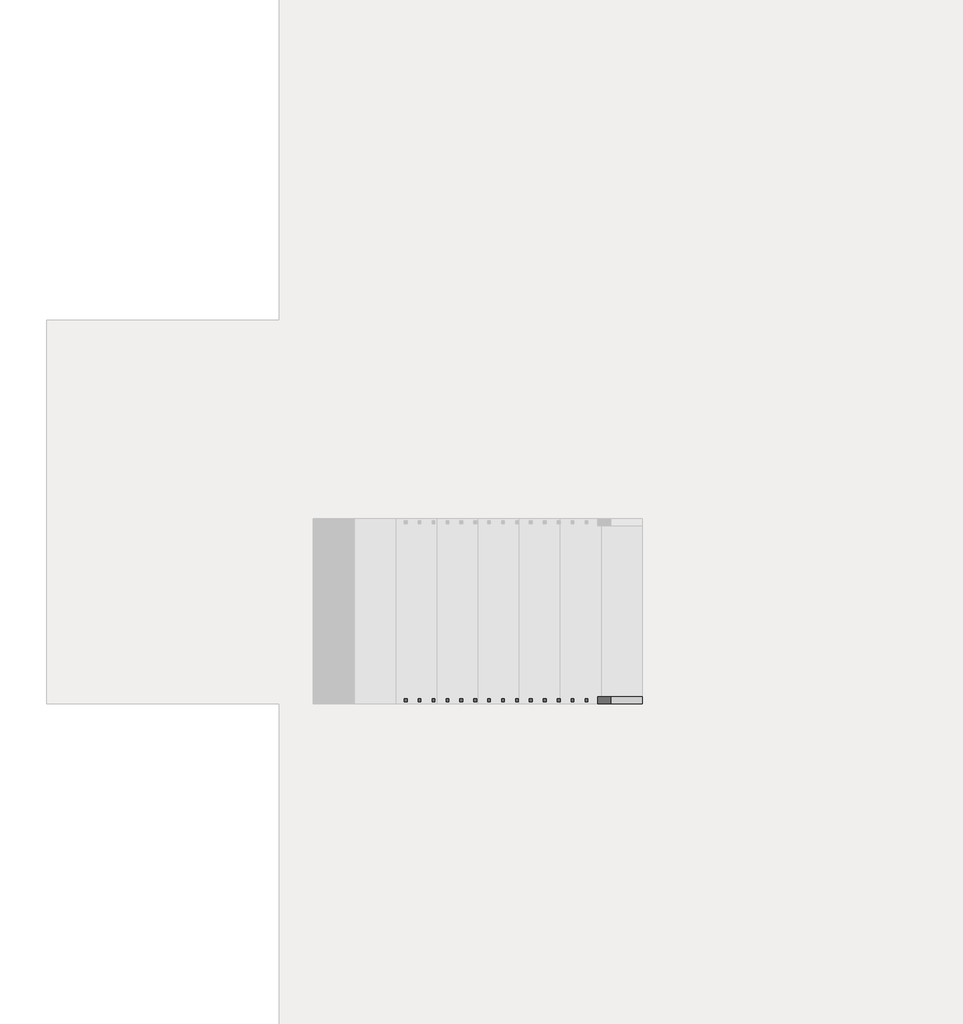
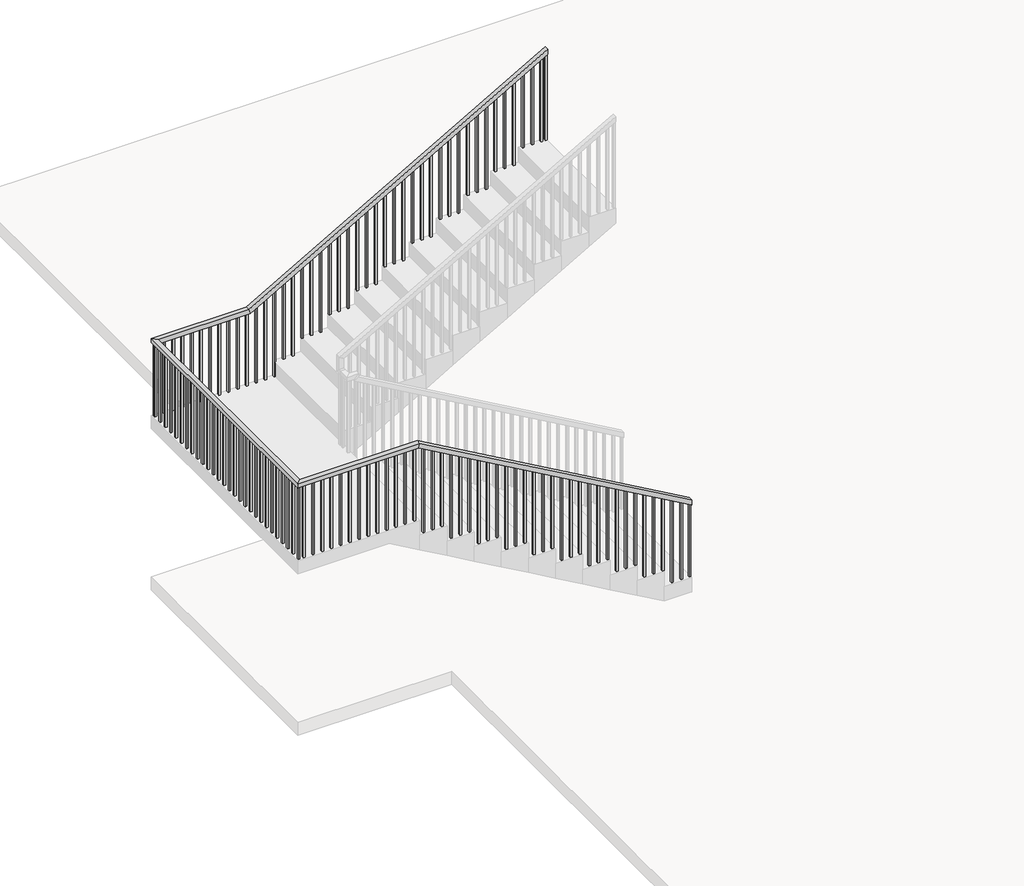
# One storey, part 2 of 3: 1 railing.
"""IFC4 building model written with IfcOpenShell, lengths in millimetres."""

from ifc_helpers import new_model, si_unit, frame, origin, place, context, project, spatial, polyline, outline, extrude, faceted_brep, element, save

model = new_model("IFC4")

# Units and contexts
model_context = context("Model", 3, world=origin())
ifc_project = project(units=[si_unit("LENGTHUNIT", "METRE", prefix="MILLI")], contexts=[model_context])

# Site, building, storey
site = spatial("IfcSite", under=ifc_project)
building = spatial("IfcBuilding", under=site)
storey = spatial("IfcBuildingStorey", under=building, Elevation=600.0)

# Railing
placement = place(None, origin())
element("IfcRailing", 1, ObjectType="Handrail - Rectangular", at=placement, inside=storey, context=model_context, shape_type="SolidModel", body=[
    faceted_brep([(-6843.9169632, -6640.1592374, 1671.4285714), (-6843.9169632, -6640.1592374, 1613.8410161), (-6843.9169632, -6590.1592374, 1613.8410161), (-6843.9169632, -6590.1592374, 1671.4285714), (-9843.9169632, -6640.1592374, 3385.7142857), (-9857.1951851, -6640.1592374, 3335.7142857), (-9857.1951851, -6590.1592374, 3335.7142857), (-9843.9169632, -6590.1592374, 3385.7142857), (-11193.5169632, -6640.1592374, 3385.7142857), (-11193.5169632, -6640.1592374, 3335.7142857), (-11143.5169632, -6590.1592374, 3335.7142857), (-11143.5169632, -6590.1592374, 3385.7142857), (-11193.5169632, -3840.9592374, 3385.7142857), (-11193.5169632, -3840.9592374, 3335.7142857), (-11143.5169632, -3890.9592374, 3335.7142857), (-11143.5169632, -3890.9592374, 3385.7142857), (-10143.9169632, -3840.9592374, 3385.7142857), (-10130.6387414, -3840.9592374, 3335.7142857), (-10130.6387414, -3890.9592374, 3335.7142857), (-10143.9169632, -3890.9592374, 3385.7142857), (-6843.9169632, -3840.9592374, 5271.4285714), (-6843.9169632, -3890.9592374, 5271.4285714), (-6843.9169632, -3890.9592374, 5213.8410161), (-6843.9169632, -3840.9592374, 5213.8410161)], [[[0, 1, 2, 3]], [[1, 0, 4, 5]], [[2, 1, 5, 6]], [[3, 2, 6, 7]], [[0, 3, 7, 4]], [[5, 4, 8, 9]], [[6, 5, 9, 10]], [[7, 6, 10, 11]], [[4, 7, 11, 8]], [[9, 8, 12, 13]], [[10, 9, 13, 14]], [[11, 10, 14, 15]], [[8, 11, 15, 12]], [[13, 12, 16, 17]], [[14, 13, 17, 18]], [[15, 14, 18, 19]], [[12, 15, 19, 16]], [[20, 21, 22, 23]], [[17, 16, 20, 23]], [[18, 17, 23, 22]], [[19, 18, 22, 21]], [[16, 19, 21, 20]]]),
    extrude(outline(polyline([(4200.0, -6911.3169632), (4200.0, -6891.3169632), (5186.7553018, -6891.3169632), (5175.3267304, -6911.3169632), (4200.0, -6911.3169632)])), frame((0.0, -3875.9592374, 0.0), z_axis=(0.0, 1.0, 0.0), x_axis=(0.0, 0.0, 1.0)), (0.0, 0.0, 1.0), 20.0),
    extrude(outline(polyline([(4200.0, -7012.9169632), (4200.0, -6992.9169632), (5128.6981589, -6992.9169632), (5117.2695875, -7012.9169632), (4200.0, -7012.9169632)])), frame((0.0, -3875.9592374, 0.0), z_axis=(0.0, 1.0, 0.0), x_axis=(0.0, 0.0, 1.0)), (0.0, 0.0, 1.0), 20.0),
    extrude(outline(polyline([(4200.0, -7114.5169632), (4200.0, -7094.5169632), (5070.6410161, -7094.5169632), (5059.2124447, -7114.5169632), (4200.0, -7114.5169632)])), frame((0.0, -3875.9592374, 0.0), z_axis=(0.0, 1.0, 0.0), x_axis=(0.0, 0.0, 1.0)), (0.0, 0.0, 1.0), 20.0),
    extrude(outline(polyline([(4028.5714286, -7216.1169632), (4028.5714286, -7196.1169632), (5012.5838732, -7196.1169632), (5001.1553018, -7216.1169632), (4028.5714286, -7216.1169632)])), frame((0.0, -3875.9592374, 0.0), z_axis=(0.0, 1.0, 0.0), x_axis=(0.0, 0.0, 1.0)), (0.0, 0.0, 1.0), 20.0),
    extrude(outline(polyline([(4028.5714286, -7317.7169632), (4028.5714286, -7297.7169632), (4954.5267304, -7297.7169632), (4943.0981589, -7317.7169632), (4028.5714286, -7317.7169632)])), frame((0.0, -3875.9592374, 0.0), z_axis=(0.0, 1.0, 0.0), x_axis=(0.0, 0.0, 1.0)), (0.0, 0.0, 1.0), 20.0),
    extrude(outline(polyline([(4028.5714286, -7419.3169632), (4028.5714286, -7399.3169632), (4896.4695875, -7399.3169632), (4885.0410161, -7419.3169632), (4028.5714286, -7419.3169632)])), frame((0.0, -3875.9592374, 0.0), z_axis=(0.0, 1.0, 0.0), x_axis=(0.0, 0.0, 1.0)), (0.0, 0.0, 1.0), 20.0),
    extrude(outline(polyline([(3857.1428571, -7520.9169632), (3857.1428571, -7500.9169632), (4838.4124447, -7500.9169632), (4826.9838732, -7520.9169632), (3857.1428571, -7520.9169632)])), frame((0.0, -3875.9592374, 0.0), z_axis=(0.0, 1.0, 0.0), x_axis=(0.0, 0.0, 1.0)), (0.0, 0.0, 1.0), 20.0),
    extrude(outline(polyline([(3857.1428571, -7622.5169632), (3857.1428571, -7602.5169632), (4780.3553018, -7602.5169632), (4768.9267304, -7622.5169632), (3857.1428571, -7622.5169632)])), frame((0.0, -3875.9592374, 0.0), z_axis=(0.0, 1.0, 0.0), x_axis=(0.0, 0.0, 1.0)), (0.0, 0.0, 1.0), 20.0),
    extrude(outline(polyline([(3857.1428571, -7724.1169632), (3857.1428571, -7704.1169632), (4722.2981589, -7704.1169632), (4710.8695875, -7724.1169632), (3857.1428571, -7724.1169632)])), frame((0.0, -3875.9592374, 0.0), z_axis=(0.0, 1.0, 0.0), x_axis=(0.0, 0.0, 1.0)), (0.0, 0.0, 1.0), 20.0),
    extrude(outline(polyline([(3685.7142857, -7825.7169632), (3685.7142857, -7805.7169632), (4664.2410161, -7805.7169632), (4652.8124447, -7825.7169632), (3685.7142857, -7825.7169632)])), frame((0.0, -3875.9592374, 0.0), z_axis=(0.0, 1.0, 0.0), x_axis=(0.0, 0.0, 1.0)), (0.0, 0.0, 1.0), 20.0),
    extrude(outline(polyline([(3685.7142857, -7927.3169632), (3685.7142857, -7907.3169632), (4606.1838732, -7907.3169632), (4594.7553018, -7927.3169632), (3685.7142857, -7927.3169632)])), frame((0.0, -3875.9592374, 0.0), z_axis=(0.0, 1.0, 0.0), x_axis=(0.0, 0.0, 1.0)), (0.0, 0.0, 1.0), 20.0),
    extrude(outline(polyline([(3685.7142857, -8028.9169632), (3685.7142857, -8008.9169632), (4548.1267304, -8008.9169632), (4536.6981589, -8028.9169632), (3685.7142857, -8028.9169632)])), frame((0.0, -3875.9592374, 0.0), z_axis=(0.0, 1.0, 0.0), x_axis=(0.0, 0.0, 1.0)), (0.0, 0.0, 1.0), 20.0),
    extrude(outline(polyline([(3514.2857143, -8130.5169632), (3514.2857143, -8110.5169632), (4490.0695875, -8110.5169632), (4478.6410161, -8130.5169632), (3514.2857143, -8130.5169632)])), frame((0.0, -3875.9592374, 0.0), z_axis=(0.0, 1.0, 0.0), x_axis=(0.0, 0.0, 1.0)), (0.0, 0.0, 1.0), 20.0),
    extrude(outline(polyline([(3514.2857143, -8232.1169632), (3514.2857143, -8212.1169632), (4432.0124447, -8212.1169632), (4420.5838732, -8232.1169632), (3514.2857143, -8232.1169632)])), frame((0.0, -3875.9592374, 0.0), z_axis=(0.0, 1.0, 0.0), x_axis=(0.0, 0.0, 1.0)), (0.0, 0.0, 1.0), 20.0),
    extrude(outline(polyline([(3514.2857143, -8333.7169632), (3514.2857143, -8313.7169632), (4373.9553018, -8313.7169632), (4362.5267304, -8333.7169632), (3514.2857143, -8333.7169632)])), frame((0.0, -3875.9592374, 0.0), z_axis=(0.0, 1.0, 0.0), x_axis=(0.0, 0.0, 1.0)), (0.0, 0.0, 1.0), 20.0),
    extrude(outline(polyline([(3342.8571429, -8435.3169632), (3342.8571429, -8415.3169632), (4315.8981589, -8415.3169632), (4304.4695875, -8435.3169632), (3342.8571429, -8435.3169632)])), frame((0.0, -3875.9592374, 0.0), z_axis=(0.0, 1.0, 0.0), x_axis=(0.0, 0.0, 1.0)), (0.0, 0.0, 1.0), 20.0),
    extrude(outline(polyline([(3342.8571429, -8536.9169632), (3342.8571429, -8516.9169632), (4257.8410161, -8516.9169632), (4246.4124447, -8536.9169632), (3342.8571429, -8536.9169632)])), frame((0.0, -3875.9592374, 0.0), z_axis=(0.0, 1.0, 0.0), x_axis=(0.0, 0.0, 1.0)), (0.0, 0.0, 1.0), 20.0),
    extrude(outline(polyline([(3342.8571429, -8638.5169632), (3342.8571429, -8618.5169632), (4199.7838732, -8618.5169632), (4188.3553018, -8638.5169632), (3342.8571429, -8638.5169632)])), frame((0.0, -3875.9592374, 0.0), z_axis=(0.0, 1.0, 0.0), x_axis=(0.0, 0.0, 1.0)), (0.0, 0.0, 1.0), 20.0),
    extrude(outline(polyline([(3171.4285714, -8740.1169632), (3171.4285714, -8720.1169632), (4141.7267304, -8720.1169632), (4130.2981589, -8740.1169632), (3171.4285714, -8740.1169632)])), frame((0.0, -3875.9592374, 0.0), z_axis=(0.0, 1.0, 0.0), x_axis=(0.0, 0.0, 1.0)), (0.0, 0.0, 1.0), 20.0),
    extrude(outline(polyline([(3171.4285714, -8841.7169632), (3171.4285714, -8821.7169632), (4083.6695875, -8821.7169632), (4072.2410161, -8841.7169632), (3171.4285714, -8841.7169632)])), frame((0.0, -3875.9592374, 0.0), z_axis=(0.0, 1.0, 0.0), x_axis=(0.0, 0.0, 1.0)), (0.0, 0.0, 1.0), 20.0),
    extrude(outline(polyline([(3171.4285714, -8943.3169632), (3171.4285714, -8923.3169632), (4025.6124447, -8923.3169632), (4014.1838732, -8943.3169632), (3171.4285714, -8943.3169632)])), frame((0.0, -3875.9592374, 0.0), z_axis=(0.0, 1.0, 0.0), x_axis=(0.0, 0.0, 1.0)), (0.0, 0.0, 1.0), 20.0),
    extrude(outline(polyline([(3000.0, -9044.9169632), (3000.0, -9024.9169632), (3967.5553018, -9024.9169632), (3956.1267304, -9044.9169632), (3000.0, -9044.9169632)])), frame((0.0, -3875.9592374, 0.0), z_axis=(0.0, 1.0, 0.0), x_axis=(0.0, 0.0, 1.0)), (0.0, 0.0, 1.0), 20.0),
    extrude(outline(polyline([(3000.0, -9146.5169632), (3000.0, -9126.5169632), (3909.4981589, -9126.5169632), (3898.0695875, -9146.5169632), (3000.0, -9146.5169632)])), frame((0.0, -3875.9592374, 0.0), z_axis=(0.0, 1.0, 0.0), x_axis=(0.0, 0.0, 1.0)), (0.0, 0.0, 1.0), 20.0),
    extrude(outline(polyline([(3000.0, -9248.1169632), (3000.0, -9228.1169632), (3851.4410161, -9228.1169632), (3840.0124447, -9248.1169632), (3000.0, -9248.1169632)])), frame((0.0, -3875.9592374, 0.0), z_axis=(0.0, 1.0, 0.0), x_axis=(0.0, 0.0, 1.0)), (0.0, 0.0, 1.0), 20.0),
    extrude(outline(polyline([(2828.5714286, -9349.7169632), (2828.5714286, -9329.7169632), (3793.3838732, -9329.7169632), (3781.9553018, -9349.7169632), (2828.5714286, -9349.7169632)])), frame((0.0, -3875.9592374, 0.0), z_axis=(0.0, 1.0, 0.0), x_axis=(0.0, 0.0, 1.0)), (0.0, 0.0, 1.0), 20.0),
    extrude(outline(polyline([(2828.5714286, -9451.3169632), (2828.5714286, -9431.3169632), (3735.3267304, -9431.3169632), (3723.8981589, -9451.3169632), (2828.5714286, -9451.3169632)])), frame((0.0, -3875.9592374, 0.0), z_axis=(0.0, 1.0, 0.0), x_axis=(0.0, 0.0, 1.0)), (0.0, 0.0, 1.0), 20.0),
    extrude(outline(polyline([(2828.5714286, -9552.9169632), (2828.5714286, -9532.9169632), (3677.2695875, -9532.9169632), (3665.8410161, -9552.9169632), (2828.5714286, -9552.9169632)])), frame((0.0, -3875.9592374, 0.0), z_axis=(0.0, 1.0, 0.0), x_axis=(0.0, 0.0, 1.0)), (0.0, 0.0, 1.0), 20.0),
    extrude(outline(polyline([(2657.1428571, -9654.5169632), (2657.1428571, -9634.5169632), (3619.2124447, -9634.5169632), (3607.7838732, -9654.5169632), (2657.1428571, -9654.5169632)])), frame((0.0, -3875.9592374, 0.0), z_axis=(0.0, 1.0, 0.0), x_axis=(0.0, 0.0, 1.0)), (0.0, 0.0, 1.0), 20.0),
    extrude(outline(polyline([(2657.1428571, -9756.1169632), (2657.1428571, -9736.1169632), (3561.1553018, -9736.1169632), (3549.7267304, -9756.1169632), (2657.1428571, -9756.1169632)])), frame((0.0, -3875.9592374, 0.0), z_axis=(0.0, 1.0, 0.0), x_axis=(0.0, 0.0, 1.0)), (0.0, 0.0, 1.0), 20.0),
    extrude(outline(polyline([(2485.7142857, -9857.7169632), (2485.7142857, -9837.7169632), (3503.0981589, -9837.7169632), (3491.6695875, -9857.7169632), (2485.7142857, -9857.7169632)])), frame((0.0, -3875.9592374, 0.0), z_axis=(0.0, 1.0, 0.0), x_axis=(0.0, 0.0, 1.0)), (0.0, 0.0, 1.0), 20.0),
    extrude(outline(polyline([(2485.7142857, -9959.3169632), (2485.7142857, -9939.3169632), (3445.0410161, -9939.3169632), (3433.6124447, -9959.3169632), (2485.7142857, -9959.3169632)])), frame((0.0, -3875.9592374, 0.0), z_axis=(0.0, 1.0, 0.0), x_axis=(0.0, 0.0, 1.0)), (0.0, 0.0, 1.0), 20.0),
    extrude(outline(polyline([(2485.7142857, -10060.9169632), (2485.7142857, -10040.9169632), (3386.9838732, -10040.9169632), (3375.5553018, -10060.9169632), (2485.7142857, -10060.9169632)])), frame((0.0, -3875.9592374, 0.0), z_axis=(0.0, 1.0, 0.0), x_axis=(0.0, 0.0, 1.0)), (0.0, 0.0, 1.0), 20.0),
    extrude(outline(polyline([(-10162.5169632, -3855.9592374), (-10142.5169632, -3855.9592374), (-10142.5169632, -3875.9592374), (-10162.5169632, -3875.9592374), (-10162.5169632, -3855.9592374)])), frame((0.0, 0.0, 2485.7142857), z_axis=(0.0, 0.0, 1.0), x_axis=(1.0, 0.0, 0.0)), (0.0, 0.0, 1.0), 850.0),
    extrude(outline(polyline([(-10264.1169632, -3855.9592374), (-10244.1169632, -3855.9592374), (-10244.1169632, -3875.9592374), (-10264.1169632, -3875.9592374), (-10264.1169632, -3855.9592374)])), frame((0.0, 0.0, 2485.7142857), z_axis=(0.0, 0.0, 1.0), x_axis=(1.0, 0.0, 0.0)), (0.0, 0.0, 1.0), 850.0),
    extrude(outline(polyline([(-10365.7169632, -3855.9592374), (-10345.7169632, -3855.9592374), (-10345.7169632, -3875.9592374), (-10365.7169632, -3875.9592374), (-10365.7169632, -3855.9592374)])), frame((0.0, 0.0, 2485.7142857), z_axis=(0.0, 0.0, 1.0), x_axis=(1.0, 0.0, 0.0)), (0.0, 0.0, 1.0), 850.0),
    extrude(outline(polyline([(-10467.3169632, -3855.9592374), (-10447.3169632, -3855.9592374), (-10447.3169632, -3875.9592374), (-10467.3169632, -3875.9592374), (-10467.3169632, -3855.9592374)])), frame((0.0, 0.0, 2485.7142857), z_axis=(0.0, 0.0, 1.0), x_axis=(1.0, 0.0, 0.0)), (0.0, 0.0, 1.0), 850.0),
    extrude(outline(polyline([(-10568.9169632, -3855.9592374), (-10548.9169632, -3855.9592374), (-10548.9169632, -3875.9592374), (-10568.9169632, -3875.9592374), (-10568.9169632, -3855.9592374)])), frame((0.0, 0.0, 2485.7142857), z_axis=(0.0, 0.0, 1.0), x_axis=(1.0, 0.0, 0.0)), (0.0, 0.0, 1.0), 850.0),
    extrude(outline(polyline([(-10670.5169632, -3855.9592374), (-10650.5169632, -3855.9592374), (-10650.5169632, -3875.9592374), (-10670.5169632, -3875.9592374), (-10670.5169632, -3855.9592374)])), frame((0.0, 0.0, 2485.7142857), z_axis=(0.0, 0.0, 1.0), x_axis=(1.0, 0.0, 0.0)), (0.0, 0.0, 1.0), 850.0),
    extrude(outline(polyline([(-10772.1169632, -3855.9592374), (-10752.1169632, -3855.9592374), (-10752.1169632, -3875.9592374), (-10772.1169632, -3875.9592374), (-10772.1169632, -3855.9592374)])), frame((0.0, 0.0, 2485.7142857), z_axis=(0.0, 0.0, 1.0), x_axis=(1.0, 0.0, 0.0)), (0.0, 0.0, 1.0), 850.0),
    extrude(outline(polyline([(-10873.7169632, -3855.9592374), (-10853.7169632, -3855.9592374), (-10853.7169632, -3875.9592374), (-10873.7169632, -3875.9592374), (-10873.7169632, -3855.9592374)])), frame((0.0, 0.0, 2485.7142857), z_axis=(0.0, 0.0, 1.0), x_axis=(1.0, 0.0, 0.0)), (0.0, 0.0, 1.0), 850.0),
    extrude(outline(polyline([(-10975.3169632, -3855.9592374), (-10955.3169632, -3855.9592374), (-10955.3169632, -3875.9592374), (-10975.3169632, -3875.9592374), (-10975.3169632, -3855.9592374)])), frame((0.0, 0.0, 2485.7142857), z_axis=(0.0, 0.0, 1.0), x_axis=(1.0, 0.0, 0.0)), (0.0, 0.0, 1.0), 850.0),
    extrude(outline(polyline([(-11076.9169632, -3855.9592374), (-11056.9169632, -3855.9592374), (-11056.9169632, -3875.9592374), (-11076.9169632, -3875.9592374), (-11076.9169632, -3855.9592374)])), frame((0.0, 0.0, 2485.7142857), z_axis=(0.0, 0.0, 1.0), x_axis=(1.0, 0.0, 0.0)), (0.0, 0.0, 1.0), 850.0),
    extrude(outline(polyline([(-11178.5169632, -3881.9592374), (-11178.5169632, -3861.9592374), (-11158.5169632, -3861.9592374), (-11158.5169632, -3881.9592374), (-11178.5169632, -3881.9592374)])), frame((0.0, 0.0, 2485.7142857), z_axis=(0.0, 0.0, 1.0), x_axis=(1.0, 0.0, 0.0)), (0.0, 0.0, 1.0), 850.0),
    extrude(outline(polyline([(-11178.5169632, -3983.5592374), (-11178.5169632, -3963.5592374), (-11158.5169632, -3963.5592374), (-11158.5169632, -3983.5592374), (-11178.5169632, -3983.5592374)])), frame((0.0, 0.0, 2485.7142857), z_axis=(0.0, 0.0, 1.0), x_axis=(1.0, 0.0, 0.0)), (0.0, 0.0, 1.0), 850.0),
    extrude(outline(polyline([(-11178.5169632, -4085.1592374), (-11178.5169632, -4065.1592374), (-11158.5169632, -4065.1592374), (-11158.5169632, -4085.1592374), (-11178.5169632, -4085.1592374)])), frame((0.0, 0.0, 2485.7142857), z_axis=(0.0, 0.0, 1.0), x_axis=(1.0, 0.0, 0.0)), (0.0, 0.0, 1.0), 850.0),
    extrude(outline(polyline([(-11178.5169632, -4186.7592374), (-11178.5169632, -4166.7592374), (-11158.5169632, -4166.7592374), (-11158.5169632, -4186.7592374), (-11178.5169632, -4186.7592374)])), frame((0.0, 0.0, 2485.7142857), z_axis=(0.0, 0.0, 1.0), x_axis=(1.0, 0.0, 0.0)), (0.0, 0.0, 1.0), 850.0),
    extrude(outline(polyline([(-11178.5169632, -4288.3592374), (-11178.5169632, -4268.3592374), (-11158.5169632, -4268.3592374), (-11158.5169632, -4288.3592374), (-11178.5169632, -4288.3592374)])), frame((0.0, 0.0, 2485.7142857), z_axis=(0.0, 0.0, 1.0), x_axis=(1.0, 0.0, 0.0)), (0.0, 0.0, 1.0), 850.0),
    extrude(outline(polyline([(-11178.5169632, -4389.9592374), (-11178.5169632, -4369.9592374), (-11158.5169632, -4369.9592374), (-11158.5169632, -4389.9592374), (-11178.5169632, -4389.9592374)])), frame((0.0, 0.0, 2485.7142857), z_axis=(0.0, 0.0, 1.0), x_axis=(1.0, 0.0, 0.0)), (0.0, 0.0, 1.0), 850.0),
    extrude(outline(polyline([(-11178.5169632, -4491.5592374), (-11178.5169632, -4471.5592374), (-11158.5169632, -4471.5592374), (-11158.5169632, -4491.5592374), (-11178.5169632, -4491.5592374)])), frame((0.0, 0.0, 2485.7142857), z_axis=(0.0, 0.0, 1.0), x_axis=(1.0, 0.0, 0.0)), (0.0, 0.0, 1.0), 850.0),
    extrude(outline(polyline([(-11178.5169632, -4593.1592374), (-11178.5169632, -4573.1592374), (-11158.5169632, -4573.1592374), (-11158.5169632, -4593.1592374), (-11178.5169632, -4593.1592374)])), frame((0.0, 0.0, 2485.7142857), z_axis=(0.0, 0.0, 1.0), x_axis=(1.0, 0.0, 0.0)), (0.0, 0.0, 1.0), 850.0),
    extrude(outline(polyline([(-11178.5169632, -4694.7592374), (-11178.5169632, -4674.7592374), (-11158.5169632, -4674.7592374), (-11158.5169632, -4694.7592374), (-11178.5169632, -4694.7592374)])), frame((0.0, 0.0, 2485.7142857), z_axis=(0.0, 0.0, 1.0), x_axis=(1.0, 0.0, 0.0)), (0.0, 0.0, 1.0), 850.0),
    extrude(outline(polyline([(-11178.5169632, -4796.3592374), (-11178.5169632, -4776.3592374), (-11158.5169632, -4776.3592374), (-11158.5169632, -4796.3592374), (-11178.5169632, -4796.3592374)])), frame((0.0, 0.0, 2485.7142857), z_axis=(0.0, 0.0, 1.0), x_axis=(1.0, 0.0, 0.0)), (0.0, 0.0, 1.0), 850.0),
    extrude(outline(polyline([(-11178.5169632, -4897.9592374), (-11178.5169632, -4877.9592374), (-11158.5169632, -4877.9592374), (-11158.5169632, -4897.9592374), (-11178.5169632, -4897.9592374)])), frame((0.0, 0.0, 2485.7142857), z_axis=(0.0, 0.0, 1.0), x_axis=(1.0, 0.0, 0.0)), (0.0, 0.0, 1.0), 850.0),
    extrude(outline(polyline([(-11178.5169632, -4999.5592374), (-11178.5169632, -4979.5592374), (-11158.5169632, -4979.5592374), (-11158.5169632, -4999.5592374), (-11178.5169632, -4999.5592374)])), frame((0.0, 0.0, 2485.7142857), z_axis=(0.0, 0.0, 1.0), x_axis=(1.0, 0.0, 0.0)), (0.0, 0.0, 1.0), 850.0),
    extrude(outline(polyline([(-11178.5169632, -5101.1592374), (-11178.5169632, -5081.1592374), (-11158.5169632, -5081.1592374), (-11158.5169632, -5101.1592374), (-11178.5169632, -5101.1592374)])), frame((0.0, 0.0, 2485.7142857), z_axis=(0.0, 0.0, 1.0), x_axis=(1.0, 0.0, 0.0)), (0.0, 0.0, 1.0), 850.0),
    extrude(outline(polyline([(-11178.5169632, -5202.7592374), (-11178.5169632, -5182.7592374), (-11158.5169632, -5182.7592374), (-11158.5169632, -5202.7592374), (-11178.5169632, -5202.7592374)])), frame((0.0, 0.0, 2485.7142857), z_axis=(0.0, 0.0, 1.0), x_axis=(1.0, 0.0, 0.0)), (0.0, 0.0, 1.0), 850.0),
    extrude(outline(polyline([(-11178.5169632, -5304.3592374), (-11178.5169632, -5284.3592374), (-11158.5169632, -5284.3592374), (-11158.5169632, -5304.3592374), (-11178.5169632, -5304.3592374)])), frame((0.0, 0.0, 2485.7142857), z_axis=(0.0, 0.0, 1.0), x_axis=(1.0, 0.0, 0.0)), (0.0, 0.0, 1.0), 850.0),
    extrude(outline(polyline([(-11178.5169632, -5405.9592374), (-11178.5169632, -5385.9592374), (-11158.5169632, -5385.9592374), (-11158.5169632, -5405.9592374), (-11178.5169632, -5405.9592374)])), frame((0.0, 0.0, 2485.7142857), z_axis=(0.0, 0.0, 1.0), x_axis=(1.0, 0.0, 0.0)), (0.0, 0.0, 1.0), 850.0),
    extrude(outline(polyline([(-11178.5169632, -5507.5592374), (-11178.5169632, -5487.5592374), (-11158.5169632, -5487.5592374), (-11158.5169632, -5507.5592374), (-11178.5169632, -5507.5592374)])), frame((0.0, 0.0, 2485.7142857), z_axis=(0.0, 0.0, 1.0), x_axis=(1.0, 0.0, 0.0)), (0.0, 0.0, 1.0), 850.0),
    extrude(outline(polyline([(-11178.5169632, -5609.1592374), (-11178.5169632, -5589.1592374), (-11158.5169632, -5589.1592374), (-11158.5169632, -5609.1592374), (-11178.5169632, -5609.1592374)])), frame((0.0, 0.0, 2485.7142857), z_axis=(0.0, 0.0, 1.0), x_axis=(1.0, 0.0, 0.0)), (0.0, 0.0, 1.0), 850.0),
    extrude(outline(polyline([(-11178.5169632, -5710.7592374), (-11178.5169632, -5690.7592374), (-11158.5169632, -5690.7592374), (-11158.5169632, -5710.7592374), (-11178.5169632, -5710.7592374)])), frame((0.0, 0.0, 2485.7142857), z_axis=(0.0, 0.0, 1.0), x_axis=(1.0, 0.0, 0.0)), (0.0, 0.0, 1.0), 850.0),
    extrude(outline(polyline([(-11178.5169632, -5812.3592374), (-11178.5169632, -5792.3592374), (-11158.5169632, -5792.3592374), (-11158.5169632, -5812.3592374), (-11178.5169632, -5812.3592374)])), frame((0.0, 0.0, 2485.7142857), z_axis=(0.0, 0.0, 1.0), x_axis=(1.0, 0.0, 0.0)), (0.0, 0.0, 1.0), 850.0),
    extrude(outline(polyline([(-11178.5169632, -5913.9592374), (-11178.5169632, -5893.9592374), (-11158.5169632, -5893.9592374), (-11158.5169632, -5913.9592374), (-11178.5169632, -5913.9592374)])), frame((0.0, 0.0, 2485.7142857), z_axis=(0.0, 0.0, 1.0), x_axis=(1.0, 0.0, 0.0)), (0.0, 0.0, 1.0), 850.0),
    extrude(outline(polyline([(-11178.5169632, -6015.5592374), (-11178.5169632, -5995.5592374), (-11158.5169632, -5995.5592374), (-11158.5169632, -6015.5592374), (-11178.5169632, -6015.5592374)])), frame((0.0, 0.0, 2485.7142857), z_axis=(0.0, 0.0, 1.0), x_axis=(1.0, 0.0, 0.0)), (0.0, 0.0, 1.0), 850.0),
    extrude(outline(polyline([(-11178.5169632, -6117.1592374), (-11178.5169632, -6097.1592374), (-11158.5169632, -6097.1592374), (-11158.5169632, -6117.1592374), (-11178.5169632, -6117.1592374)])), frame((0.0, 0.0, 2485.7142857), z_axis=(0.0, 0.0, 1.0), x_axis=(1.0, 0.0, 0.0)), (0.0, 0.0, 1.0), 850.0),
    extrude(outline(polyline([(-11178.5169632, -6218.7592374), (-11178.5169632, -6198.7592374), (-11158.5169632, -6198.7592374), (-11158.5169632, -6218.7592374), (-11178.5169632, -6218.7592374)])), frame((0.0, 0.0, 2485.7142857), z_axis=(0.0, 0.0, 1.0), x_axis=(1.0, 0.0, 0.0)), (0.0, 0.0, 1.0), 850.0),
    extrude(outline(polyline([(-11178.5169632, -6320.3592374), (-11178.5169632, -6300.3592374), (-11158.5169632, -6300.3592374), (-11158.5169632, -6320.3592374), (-11178.5169632, -6320.3592374)])), frame((0.0, 0.0, 2485.7142857), z_axis=(0.0, 0.0, 1.0), x_axis=(1.0, 0.0, 0.0)), (0.0, 0.0, 1.0), 850.0),
    extrude(outline(polyline([(-11178.5169632, -6421.9592374), (-11178.5169632, -6401.9592374), (-11158.5169632, -6401.9592374), (-11158.5169632, -6421.9592374), (-11178.5169632, -6421.9592374)])), frame((0.0, 0.0, 2485.7142857), z_axis=(0.0, 0.0, 1.0), x_axis=(1.0, 0.0, 0.0)), (0.0, 0.0, 1.0), 850.0),
    extrude(outline(polyline([(-11178.5169632, -6523.5592374), (-11178.5169632, -6503.5592374), (-11158.5169632, -6503.5592374), (-11158.5169632, -6523.5592374), (-11178.5169632, -6523.5592374)])), frame((0.0, 0.0, 2485.7142857), z_axis=(0.0, 0.0, 1.0), x_axis=(1.0, 0.0, 0.0)), (0.0, 0.0, 1.0), 850.0),
    extrude(outline(polyline([(-11101.1169632, -6625.1592374), (-11121.1169632, -6625.1592374), (-11121.1169632, -6605.1592374), (-11101.1169632, -6605.1592374), (-11101.1169632, -6625.1592374)])), frame((0.0, 0.0, 2485.7142857), z_axis=(0.0, 0.0, 1.0), x_axis=(1.0, 0.0, 0.0)), (0.0, 0.0, 1.0), 850.0),
    extrude(outline(polyline([(-10999.5169632, -6625.1592374), (-11019.5169632, -6625.1592374), (-11019.5169632, -6605.1592374), (-10999.5169632, -6605.1592374), (-10999.5169632, -6625.1592374)])), frame((0.0, 0.0, 2485.7142857), z_axis=(0.0, 0.0, 1.0), x_axis=(1.0, 0.0, 0.0)), (0.0, 0.0, 1.0), 850.0),
    extrude(outline(polyline([(-10897.9169632, -6625.1592374), (-10917.9169632, -6625.1592374), (-10917.9169632, -6605.1592374), (-10897.9169632, -6605.1592374), (-10897.9169632, -6625.1592374)])), frame((0.0, 0.0, 2485.7142857), z_axis=(0.0, 0.0, 1.0), x_axis=(1.0, 0.0, 0.0)), (0.0, 0.0, 1.0), 850.0),
    extrude(outline(polyline([(-10796.3169632, -6625.1592374), (-10816.3169632, -6625.1592374), (-10816.3169632, -6605.1592374), (-10796.3169632, -6605.1592374), (-10796.3169632, -6625.1592374)])), frame((0.0, 0.0, 2485.7142857), z_axis=(0.0, 0.0, 1.0), x_axis=(1.0, 0.0, 0.0)), (0.0, 0.0, 1.0), 850.0),
    extrude(outline(polyline([(-10694.7169632, -6625.1592374), (-10714.7169632, -6625.1592374), (-10714.7169632, -6605.1592374), (-10694.7169632, -6605.1592374), (-10694.7169632, -6625.1592374)])), frame((0.0, 0.0, 2485.7142857), z_axis=(0.0, 0.0, 1.0), x_axis=(1.0, 0.0, 0.0)), (0.0, 0.0, 1.0), 850.0),
    extrude(outline(polyline([(-10593.1169632, -6625.1592374), (-10613.1169632, -6625.1592374), (-10613.1169632, -6605.1592374), (-10593.1169632, -6605.1592374), (-10593.1169632, -6625.1592374)])), frame((0.0, 0.0, 2485.7142857), z_axis=(0.0, 0.0, 1.0), x_axis=(1.0, 0.0, 0.0)), (0.0, 0.0, 1.0), 850.0),
    extrude(outline(polyline([(-10491.5169632, -6625.1592374), (-10511.5169632, -6625.1592374), (-10511.5169632, -6605.1592374), (-10491.5169632, -6605.1592374), (-10491.5169632, -6625.1592374)])), frame((0.0, 0.0, 2485.7142857), z_axis=(0.0, 0.0, 1.0), x_axis=(1.0, 0.0, 0.0)), (0.0, 0.0, 1.0), 850.0),
    extrude(outline(polyline([(-10389.9169632, -6625.1592374), (-10409.9169632, -6625.1592374), (-10409.9169632, -6605.1592374), (-10389.9169632, -6605.1592374), (-10389.9169632, -6625.1592374)])), frame((0.0, 0.0, 2485.7142857), z_axis=(0.0, 0.0, 1.0), x_axis=(1.0, 0.0, 0.0)), (0.0, 0.0, 1.0), 850.0),
    extrude(outline(polyline([(-10288.3169632, -6625.1592374), (-10308.3169632, -6625.1592374), (-10308.3169632, -6605.1592374), (-10288.3169632, -6605.1592374), (-10288.3169632, -6625.1592374)])), frame((0.0, 0.0, 2485.7142857), z_axis=(0.0, 0.0, 1.0), x_axis=(1.0, 0.0, 0.0)), (0.0, 0.0, 1.0), 850.0),
    extrude(outline(polyline([(-10186.7169632, -6625.1592374), (-10206.7169632, -6625.1592374), (-10206.7169632, -6605.1592374), (-10186.7169632, -6605.1592374), (-10186.7169632, -6625.1592374)])), frame((0.0, 0.0, 2485.7142857), z_axis=(0.0, 0.0, 1.0), x_axis=(1.0, 0.0, 0.0)), (0.0, 0.0, 1.0), 850.0),
    extrude(outline(polyline([(-10085.1169632, -6625.1592374), (-10105.1169632, -6625.1592374), (-10105.1169632, -6605.1592374), (-10085.1169632, -6605.1592374), (-10085.1169632, -6625.1592374)])), frame((0.0, 0.0, 2485.7142857), z_axis=(0.0, 0.0, 1.0), x_axis=(1.0, 0.0, 0.0)), (0.0, 0.0, 1.0), 850.0),
    extrude(outline(polyline([(-9983.5169632, -6625.1592374), (-10003.5169632, -6625.1592374), (-10003.5169632, -6605.1592374), (-9983.5169632, -6605.1592374), (-9983.5169632, -6625.1592374)])), frame((0.0, 0.0, 2485.7142857), z_axis=(0.0, 0.0, 1.0), x_axis=(1.0, 0.0, 0.0)), (0.0, 0.0, 1.0), 850.0),
    extrude(outline(polyline([(-9881.9169632, -6625.1592374), (-9901.9169632, -6625.1592374), (-9901.9169632, -6605.1592374), (-9881.9169632, -6605.1592374), (-9881.9169632, -6625.1592374)])), frame((0.0, 0.0, 2485.7142857), z_axis=(0.0, 0.0, 1.0), x_axis=(1.0, 0.0, 0.0)), (0.0, 0.0, 1.0), 850.0),
    extrude(outline(polyline([(3291.7838732, -9780.3169632), (3303.2124447, -9800.3169632), (2314.2857143, -9800.3169632), (2314.2857143, -9780.3169632), (3291.7838732, -9780.3169632)])), frame((0.0, -6625.1592374, 0.0), z_axis=(0.0, 1.0, 0.0), x_axis=(0.0, 0.0, 1.0)), (0.0, 0.0, 1.0), 20.0),
    extrude(outline(polyline([(3233.7267304, -9678.7169632), (3245.1553018, -9698.7169632), (2314.2857143, -9698.7169632), (2314.2857143, -9678.7169632), (3233.7267304, -9678.7169632)])), frame((0.0, -6625.1592374, 0.0), z_axis=(0.0, 1.0, 0.0), x_axis=(0.0, 0.0, 1.0)), (0.0, 0.0, 1.0), 20.0),
    extrude(outline(polyline([(3175.6695875, -9577.1169632), (3187.0981589, -9597.1169632), (2314.2857143, -9597.1169632), (2314.2857143, -9577.1169632), (3175.6695875, -9577.1169632)])), frame((0.0, -6625.1592374, 0.0), z_axis=(0.0, 1.0, 0.0), x_axis=(0.0, 0.0, 1.0)), (0.0, 0.0, 1.0), 20.0),
    extrude(outline(polyline([(3117.6124447, -9475.5169632), (3129.0410161, -9495.5169632), (2142.8571429, -9495.5169632), (2142.8571429, -9475.5169632), (3117.6124447, -9475.5169632)])), frame((0.0, -6625.1592374, 0.0), z_axis=(0.0, 1.0, 0.0), x_axis=(0.0, 0.0, 1.0)), (0.0, 0.0, 1.0), 20.0),
    extrude(outline(polyline([(3059.5553018, -9373.9169632), (3070.9838732, -9393.9169632), (2142.8571429, -9393.9169632), (2142.8571429, -9373.9169632), (3059.5553018, -9373.9169632)])), frame((0.0, -6625.1592374, 0.0), z_axis=(0.0, 1.0, 0.0), x_axis=(0.0, 0.0, 1.0)), (0.0, 0.0, 1.0), 20.0),
    extrude(outline(polyline([(3001.4981589, -9272.3169632), (3012.9267304, -9292.3169632), (2142.8571429, -9292.3169632), (2142.8571429, -9272.3169632), (3001.4981589, -9272.3169632)])), frame((0.0, -6625.1592374, 0.0), z_axis=(0.0, 1.0, 0.0), x_axis=(0.0, 0.0, 1.0)), (0.0, 0.0, 1.0), 20.0),
    extrude(outline(polyline([(2943.4410161, -9170.7169632), (2954.8695875, -9190.7169632), (1971.4285714, -9190.7169632), (1971.4285714, -9170.7169632), (2943.4410161, -9170.7169632)])), frame((0.0, -6625.1592374, 0.0), z_axis=(0.0, 1.0, 0.0), x_axis=(0.0, 0.0, 1.0)), (0.0, 0.0, 1.0), 20.0),
    extrude(outline(polyline([(2885.3838732, -9069.1169632), (2896.8124447, -9089.1169632), (1971.4285714, -9089.1169632), (1971.4285714, -9069.1169632), (2885.3838732, -9069.1169632)])), frame((0.0, -6625.1592374, 0.0), z_axis=(0.0, 1.0, 0.0), x_axis=(0.0, 0.0, 1.0)), (0.0, 0.0, 1.0), 20.0),
    extrude(outline(polyline([(2827.3267304, -8967.5169632), (2838.7553018, -8987.5169632), (1971.4285714, -8987.5169632), (1971.4285714, -8967.5169632), (2827.3267304, -8967.5169632)])), frame((0.0, -6625.1592374, 0.0), z_axis=(0.0, 1.0, 0.0), x_axis=(0.0, 0.0, 1.0)), (0.0, 0.0, 1.0), 20.0),
    extrude(outline(polyline([(2769.2695875, -8865.9169632), (2780.6981589, -8885.9169632), (1800.0, -8885.9169632), (1800.0, -8865.9169632), (2769.2695875, -8865.9169632)])), frame((0.0, -6625.1592374, 0.0), z_axis=(0.0, 1.0, 0.0), x_axis=(0.0, 0.0, 1.0)), (0.0, 0.0, 1.0), 20.0),
    extrude(outline(polyline([(2711.2124447, -8764.3169632), (2722.6410161, -8784.3169632), (1800.0, -8784.3169632), (1800.0, -8764.3169632), (2711.2124447, -8764.3169632)])), frame((0.0, -6625.1592374, 0.0), z_axis=(0.0, 1.0, 0.0), x_axis=(0.0, 0.0, 1.0)), (0.0, 0.0, 1.0), 20.0),
    extrude(outline(polyline([(2653.1553018, -8662.7169632), (2664.5838732, -8682.7169632), (1800.0, -8682.7169632), (1800.0, -8662.7169632), (2653.1553018, -8662.7169632)])), frame((0.0, -6625.1592374, 0.0), z_axis=(0.0, 1.0, 0.0), x_axis=(0.0, 0.0, 1.0)), (0.0, 0.0, 1.0), 20.0),
    extrude(outline(polyline([(2595.0981589, -8561.1169632), (2606.5267304, -8581.1169632), (1628.5714286, -8581.1169632), (1628.5714286, -8561.1169632), (2595.0981589, -8561.1169632)])), frame((0.0, -6625.1592374, 0.0), z_axis=(0.0, 1.0, 0.0), x_axis=(0.0, 0.0, 1.0)), (0.0, 0.0, 1.0), 20.0),
    extrude(outline(polyline([(2537.0410161, -8459.5169632), (2548.4695875, -8479.5169632), (1628.5714286, -8479.5169632), (1628.5714286, -8459.5169632), (2537.0410161, -8459.5169632)])), frame((0.0, -6625.1592374, 0.0), z_axis=(0.0, 1.0, 0.0), x_axis=(0.0, 0.0, 1.0)), (0.0, 0.0, 1.0), 20.0),
    extrude(outline(polyline([(2478.9838732, -8357.9169632), (2490.4124447, -8377.9169632), (1628.5714286, -8377.9169632), (1628.5714286, -8357.9169632), (2478.9838732, -8357.9169632)])), frame((0.0, -6625.1592374, 0.0), z_axis=(0.0, 1.0, 0.0), x_axis=(0.0, 0.0, 1.0)), (0.0, 0.0, 1.0), 20.0),
    extrude(outline(polyline([(2420.9267304, -8256.3169632), (2432.3553018, -8276.3169632), (1457.1428571, -8276.3169632), (1457.1428571, -8256.3169632), (2420.9267304, -8256.3169632)])), frame((0.0, -6625.1592374, 0.0), z_axis=(0.0, 1.0, 0.0), x_axis=(0.0, 0.0, 1.0)), (0.0, 0.0, 1.0), 20.0),
    extrude(outline(polyline([(2362.8695875, -8154.7169632), (2374.2981589, -8174.7169632), (1457.1428571, -8174.7169632), (1457.1428571, -8154.7169632), (2362.8695875, -8154.7169632)])), frame((0.0, -6625.1592374, 0.0), z_axis=(0.0, 1.0, 0.0), x_axis=(0.0, 0.0, 1.0)), (0.0, 0.0, 1.0), 20.0),
    extrude(outline(polyline([(2304.8124447, -8053.1169632), (2316.2410161, -8073.1169632), (1457.1428571, -8073.1169632), (1457.1428571, -8053.1169632), (2304.8124447, -8053.1169632)])), frame((0.0, -6625.1592374, 0.0), z_axis=(0.0, 1.0, 0.0), x_axis=(0.0, 0.0, 1.0)), (0.0, 0.0, 1.0), 20.0),
    extrude(outline(polyline([(2246.7553018, -7951.5169632), (2258.1838732, -7971.5169632), (1285.7142857, -7971.5169632), (1285.7142857, -7951.5169632), (2246.7553018, -7951.5169632)])), frame((0.0, -6625.1592374, 0.0), z_axis=(0.0, 1.0, 0.0), x_axis=(0.0, 0.0, 1.0)), (0.0, 0.0, 1.0), 20.0),
    extrude(outline(polyline([(2188.6981589, -7849.9169632), (2200.1267304, -7869.9169632), (1285.7142857, -7869.9169632), (1285.7142857, -7849.9169632), (2188.6981589, -7849.9169632)])), frame((0.0, -6625.1592374, 0.0), z_axis=(0.0, 1.0, 0.0), x_axis=(0.0, 0.0, 1.0)), (0.0, 0.0, 1.0), 20.0),
    extrude(outline(polyline([(2130.6410161, -7748.3169632), (2142.0695875, -7768.3169632), (1285.7142857, -7768.3169632), (1285.7142857, -7748.3169632), (2130.6410161, -7748.3169632)])), frame((0.0, -6625.1592374, 0.0), z_axis=(0.0, 1.0, 0.0), x_axis=(0.0, 0.0, 1.0)), (0.0, 0.0, 1.0), 20.0),
    extrude(outline(polyline([(2072.5838732, -7646.7169632), (2084.0124447, -7666.7169632), (1114.2857143, -7666.7169632), (1114.2857143, -7646.7169632), (2072.5838732, -7646.7169632)])), frame((0.0, -6625.1592374, 0.0), z_axis=(0.0, 1.0, 0.0), x_axis=(0.0, 0.0, 1.0)), (0.0, 0.0, 1.0), 20.0),
    extrude(outline(polyline([(2014.5267304, -7545.1169632), (2025.9553018, -7565.1169632), (1114.2857143, -7565.1169632), (1114.2857143, -7545.1169632), (2014.5267304, -7545.1169632)])), frame((0.0, -6625.1592374, 0.0), z_axis=(0.0, 1.0, 0.0), x_axis=(0.0, 0.0, 1.0)), (0.0, 0.0, 1.0), 20.0),
    extrude(outline(polyline([(1956.4124447, -7443.5169632), (1967.8410161, -7463.5169632), (1114.2857143, -7463.5169632), (1114.2857143, -7443.5169632), (1956.4124447, -7443.5169632)])), frame((0.0, -6625.1592374, 0.0), z_axis=(0.0, 1.0, 0.0), x_axis=(0.0, 0.0, 1.0)), (0.0, 0.0, 1.0), 20.0),
    extrude(outline(polyline([(1898.4124447, -7341.9169632), (1909.8410161, -7361.9169632), (942.8571429, -7361.9169632), (942.8571429, -7341.9169632), (1898.4124447, -7341.9169632)])), frame((0.0, -6625.1592374, 0.0), z_axis=(0.0, 1.0, 0.0), x_axis=(0.0, 0.0, 1.0)), (0.0, 0.0, 1.0), 20.0),
    extrude(outline(polyline([(1840.3553018, -7240.3169632), (1851.7838732, -7260.3169632), (942.8571429, -7260.3169632), (942.8571429, -7240.3169632), (1840.3553018, -7240.3169632)])), frame((0.0, -6625.1592374, 0.0), z_axis=(0.0, 1.0, 0.0), x_axis=(0.0, 0.0, 1.0)), (0.0, 0.0, 1.0), 20.0),
    extrude(outline(polyline([(1782.2981589, -7138.7169632), (1793.7267304, -7158.7169632), (942.8571429, -7158.7169632), (942.8571429, -7138.7169632), (1782.2981589, -7138.7169632)])), frame((0.0, -6625.1592374, 0.0), z_axis=(0.0, 1.0, 0.0), x_axis=(0.0, 0.0, 1.0)), (0.0, 0.0, 1.0), 20.0),
    extrude(outline(polyline([(1724.2410161, -7037.1169632), (1735.6695875, -7057.1169632), (771.4285714, -7057.1169632), (771.4285714, -7037.1169632), (1724.2410161, -7037.1169632)])), frame((0.0, -6625.1592374, 0.0), z_axis=(0.0, 1.0, 0.0), x_axis=(0.0, 0.0, 1.0)), (0.0, 0.0, 1.0), 20.0),
    extrude(outline(polyline([(1666.1838732, -6935.5169632), (1677.6124447, -6955.5169632), (771.4285714, -6955.5169632), (771.4285714, -6935.5169632), (1666.1838732, -6935.5169632)])), frame((0.0, -6625.1592374, 0.0), z_axis=(0.0, 1.0, 0.0), x_axis=(0.0, 0.0, 1.0)), (0.0, 0.0, 1.0), 20.0),
    extrude(outline(polyline([(-11178.5169632, -3875.9592374), (-11178.5169632, -3855.9592374), (-11158.5169632, -3855.9592374), (-11158.5169632, -3875.9592374), (-11178.5169632, -3875.9592374)])), frame((0.0, 0.0, 2485.7142857), z_axis=(0.0, 0.0, 1.0), x_axis=(1.0, 0.0, 0.0)), (0.0, 0.0, 1.0), 850.0),
    extrude(outline(polyline([(-11158.5169632, -6625.1592374), (-11178.5169632, -6625.1592374), (-11178.5169632, -6605.1592374), (-11158.5169632, -6605.1592374), (-11158.5169632, -6625.1592374)])), frame((0.0, 0.0, 2485.7142857), z_axis=(0.0, 0.0, 1.0), x_axis=(1.0, 0.0, 0.0)), (0.0, 0.0, 1.0), 850.0),
    extrude(outline(polyline([(4200.0, -6863.4169632), (4200.0, -6843.4169632), (5214.1267304, -6843.4169632), (5202.6981589, -6863.4169632), (4200.0, -6863.4169632)])), frame((0.0, -3875.9592374, 0.0), z_axis=(0.0, 1.0, 0.0), x_axis=(0.0, 0.0, 1.0)), (0.0, 0.0, 1.0), 20.0),
    extrude(outline(polyline([(1613.5553018, -6843.4169632), (1624.9838732, -6863.4169632), (771.4285714, -6863.4169632), (771.4285714, -6843.4169632), (1613.5553018, -6843.4169632)])), frame((0.0, -6625.1592374, 0.0), z_axis=(0.0, 1.0, 0.0), x_axis=(0.0, 0.0, 1.0)), (0.0, 0.0, 1.0), 20.0),
])

save(model, "model.ifc")

# Revit data of these elements
# Type "Handrail - Rectangular"
#   Assembly Code = "C2010400"
#   built-in parameter 1008612 = 0.0416667 (stored number, unit not read)
#   built-in parameter 1008611 = 0.0416667 (stored number, unit not read)
#   built-in parameter 1008609 = 0.333333 (stored number, unit not read)
#   built-in parameter 1008604 = 0.166667 (stored number, unit not read)
#   built-in parameter 1008603 = 0.166667 (stored number, unit not read)
#   Railing Height = 900 mm
#   built-in parameter 1008630 = 2
#   built-in parameter 1008610 = 2
# Element 1 (IfcRailing, "Handrail - Rectangular")
#   Phase Created = New Construction
